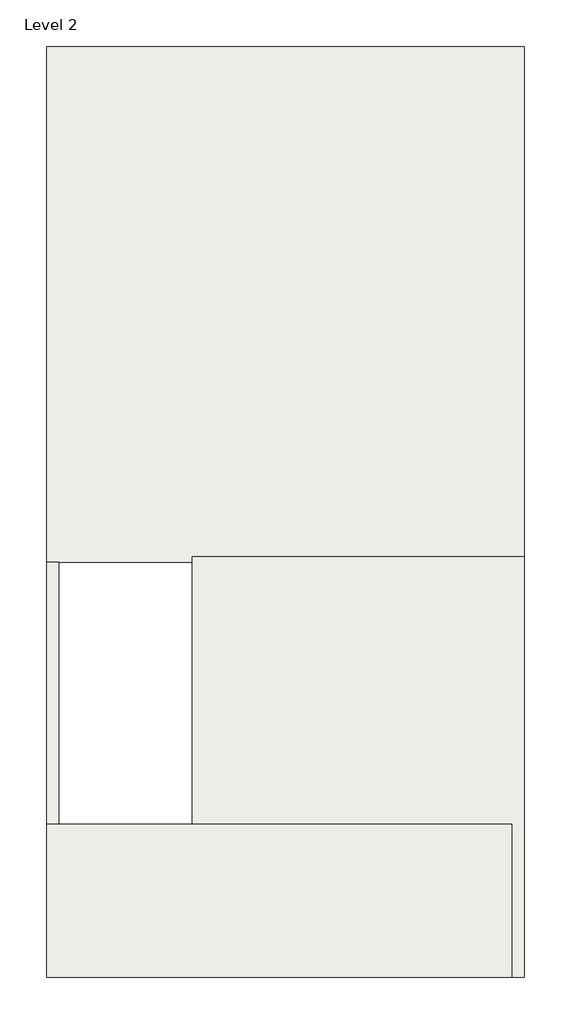
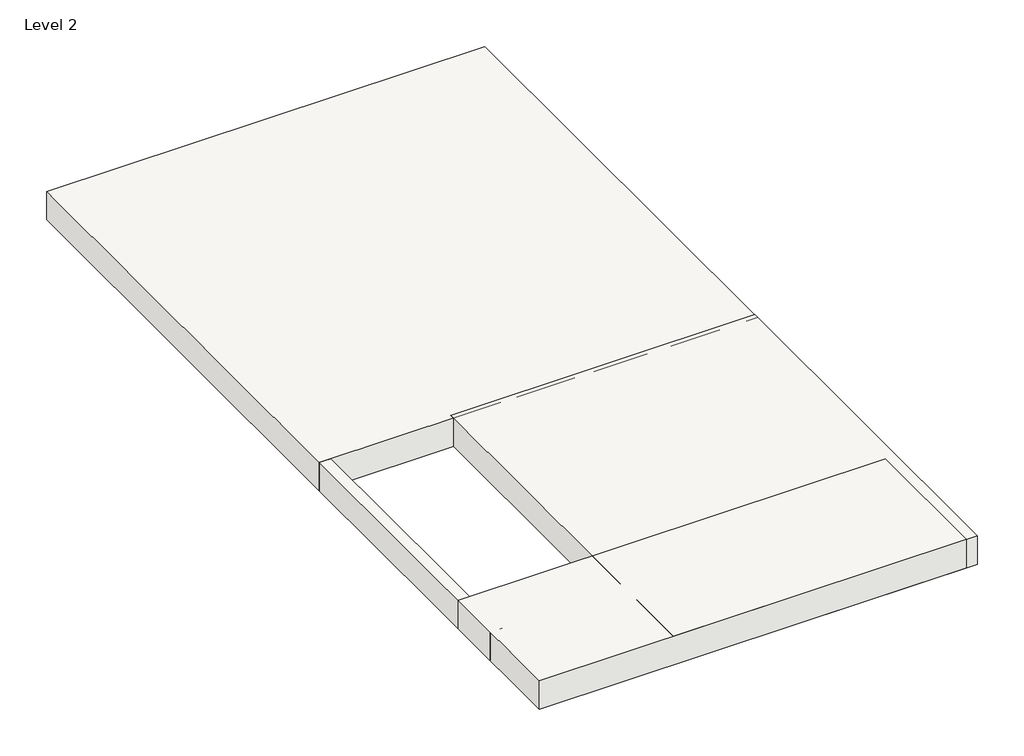
# One storey: 4 roofs.
"""IFC4 building model written with IfcOpenShell, lengths in millimetres."""

from ifc_helpers import new_model, si_unit, frame, origin, place, context, project, spatial, polyline, outline, extrude, element, save

model = new_model("IFC4")

# Units and contexts
model_context = context("Model", 3, world=origin())
ifc_project = project(units=[si_unit("LENGTHUNIT", "METRE", prefix="MILLI")], contexts=[model_context])

# Site, building, storey
site = spatial("IfcSite", under=ifc_project)
building = spatial("IfcBuilding", under=site)
storey = spatial("IfcBuildingStorey", under=building, Name="Level 2", Elevation=3048.0)

# Roofs
placement = place(None, origin())
element("IfcRoof", 1, ObjectType="Steel Truss - Insulation on Metal Deck - EPDM", at=placement, inside=storey, context=model_context, shape_type="SweptSolid", body=[
    extrude(outline(polyline([(-13564.5568901, 13670.121124), (-5563.5568901, 13670.121124), (-5563.5568901, 5034.121124), (-13564.5568901, 5034.121124), (-13564.5568901, 13670.121124)])), frame((0.0, 0.0, 3048.0), z_axis=(0.0, 0.0, 1.0), x_axis=(1.0, 0.0, 0.0)), (0.0, 0.0, 1.0), 546.1),
])
element("IfcRoof", 2, ObjectType="Steel Truss - Insulation on Metal Deck - EPDM", at=placement, inside=storey, context=model_context, shape_type="SweptSolid", body=[
    extrude(outline(polyline([(-11119.8068901, -1925.478876), (-11119.8068901, 5123.021124), (-5563.5568901, 5123.021124), (-5563.5568901, -1925.478876), (-11119.8068901, -1925.478876)])), frame((0.0, 0.0, 3048.0), z_axis=(0.0, 0.0, 1.0), x_axis=(1.0, 0.0, 0.0)), (0.0, 0.0, 1.0), 546.1),
])
element("IfcRoof", 3, ObjectType="Steel Truss - Insulation on Metal Deck - EPDM", at=placement, inside=storey, context=model_context, shape_type="SweptSolid", body=[
    extrude(outline(polyline([(-13564.5568901, 639.921124), (-5766.7568901, 639.921124), (-5766.7568901, -1925.478876), (-13564.5568901, -1925.478876), (-13564.5568901, 639.921124)])), frame((0.0, 0.0, 3048.0), z_axis=(0.0, 0.0, 1.0), x_axis=(1.0, 0.0, 0.0)), (0.0, 0.0, 1.0), 546.1),
])
element("IfcRoof", 4, ObjectType="Steel Truss - Insulation on Metal Deck - EPDM", at=placement, inside=storey, context=model_context, shape_type="SweptSolid", body=[
    extrude(outline(polyline([(-13564.5568901, -376.078876), (-13564.5568901, 5034.121124), (-13361.3568901, 5034.121124), (-13361.3568901, -376.078876), (-13462.9568901, -376.078876), (-13564.5568901, -376.078876)])), frame((0.0, 0.0, 3048.0), z_axis=(0.0, 0.0, 1.0), x_axis=(1.0, 0.0, 0.0)), (0.0, 0.0, 1.0), 546.1),
])

save(model, "model.ifc")

# Revit data of these elements
# Type "Steel Truss - Insulation on Metal Deck - EPDM"
#   Assembly Code = "B1020"
#   Layers, outside or top first: 0' - 0 1/4" "Roofing, EPDM Membrane" (function 4); 0' - 5" "Rigid insulation" (function 3); 0' - 0 1/4" "Metal Deck" (function 1); 1' - 4" "Structure, Steel Bar Joist Layer" (function 1)
# Elements 1, 2, 3, 4 (IfcRoof, "Steel Truss - Insulation on Metal Deck - EPDM")
#   built-in parameter 1001705 = 11.7917 (stored number, unit not read)
#   built-in parameter 1001710 = 33615
#   Phase Created = New Construction
#   Materials on its faces: "Structure, Steel Bar Joist Layer", "Roofing, EPDM Membrane"
# Materials
#   "Roofing, EPDM Membrane": class "Generic", colour RGB 127 127 127, transparency 0, Description = "EPDM roof membrane", Cost = 0
#   "Rigid insulation": class "Generic", colour RGB 127 127 127, transparency 0, Description = "Rigid foam insulation board", Cost = 0
#   "Metal Deck": class "Metal", colour RGB 199 199 199, transparency 0, Description = "Steel, mill finish", Cost = 0
#   "Structure, Steel Bar Joist Layer": class "Metal", colour RGB 127 127 127, transparency 0, Description = "Bar joists, thermal airspace", Cost = 0
